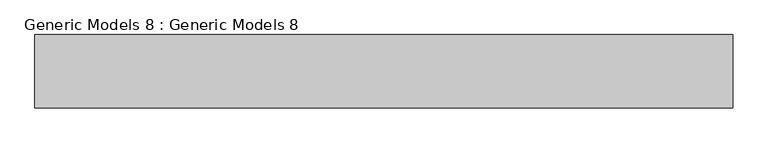
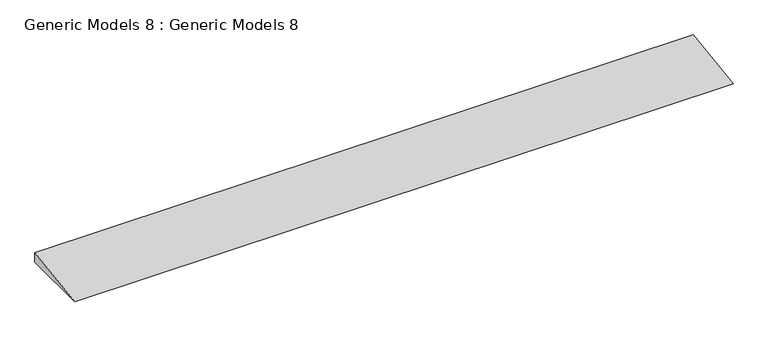
"""IFC4 building model written with IfcOpenShell, lengths in millimetres: proxy geometry, Generic Models 8 : Generic Models 8."""

from ifc_helpers import new_model, si_unit, frame, origin, place, context, project, spatial, polyline, outline, extrude, source, transform, mapped, element, save


def generic_models_8_generic_models_8_37e38eb9(model_context):
    return source(origin(), model_context, "Body", "SweptSolid", [
        extrude(outline(polyline([(-8942.7038063, -152.4), (-7860.0977377, 0.0), (-7860.0977377, -152.4), (-8942.7038063, -152.4)])), frame((-3622.8563205, 0.0, 0.0), z_axis=(1.0, 0.0, 0.0), x_axis=(0.0, 1.0, 0.0)), (0.0, 0.0, 1.0), 10292.4148121),
    ])


if __name__ == "__main__":
    model = new_model("IFC4")
    model_context = context("Model", 3, world=origin())
    ifc_project = project(units=[si_unit("LENGTHUNIT", "METRE", prefix="MILLI")], contexts=[model_context])
    site = spatial("IfcSite", under=ifc_project)
    building = spatial("IfcBuilding", under=site)
    placement = place(None, origin())
    generic_models_8_generic_models_8_shape = generic_models_8_generic_models_8_37e38eb9(model_context)
    element("IfcBuildingElementProxy", 1, Name="Generic Models 8 : Generic Models 8", ObjectType="Generic Models 8 : Generic Models 8", at=placement, inside=building, context=model_context, shape_type="MappedRepresentation", body=[
        mapped(generic_models_8_generic_models_8_shape, transform((0.0, 0.0, 0.0), x_axis=(1.0, 0.0, 0.0), y_axis=(0.0, 1.0, 0.0), z_axis=(0.0, 0.0, 1.0))),
    ])
    save(model, "model.ifc")
